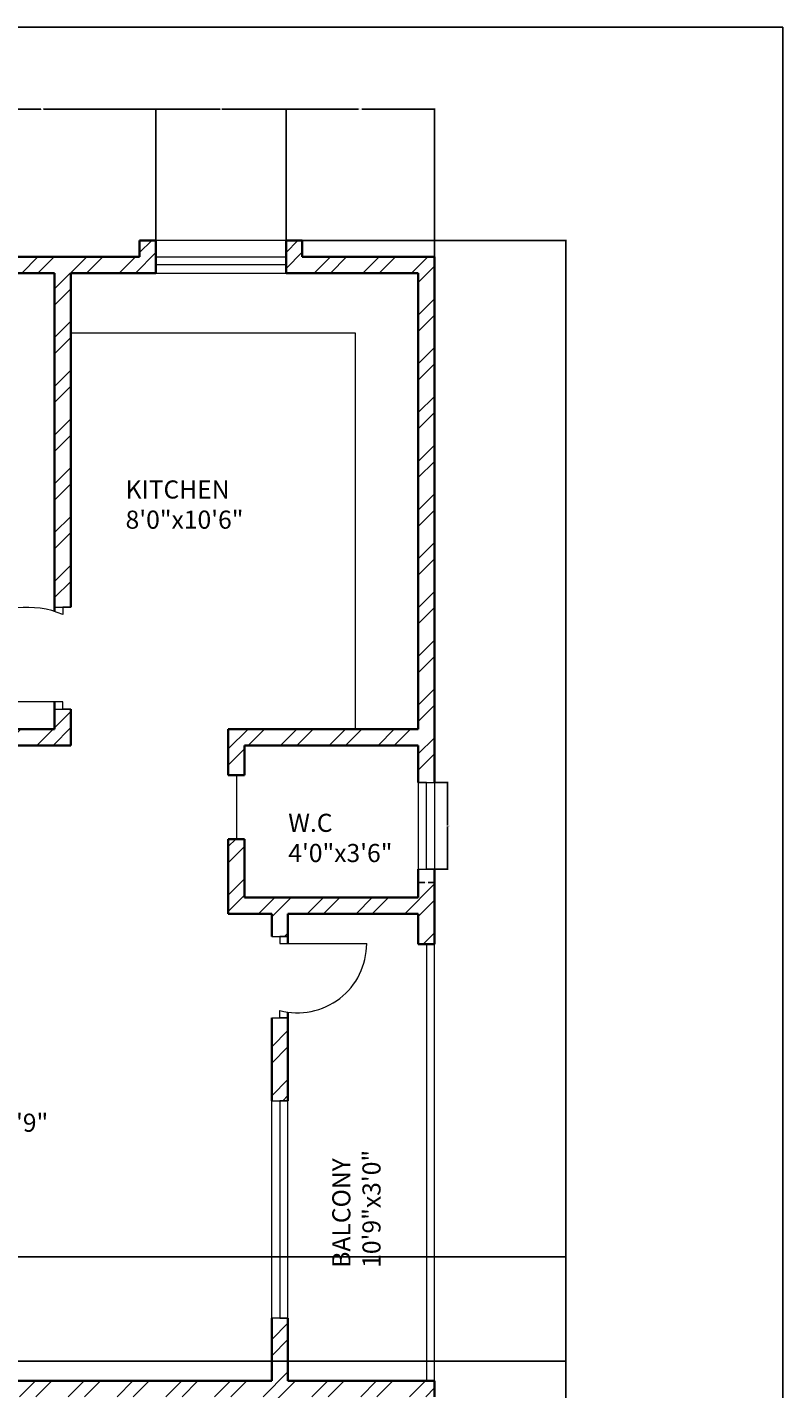
# Model space of a CAD drawing. Units: inches. Extents: x 1570 to 2186, y 1575 to 2421.
# Tile 10 of 10: x 1978 to 2186, y 2045 to 2421. Entities that reach past the tile are written whole.
import ezdxf

# ---------------------------------------------------------------- set-up
doc = ezdxf.new("R2010")
doc.units = ezdxf.units.IN
for name, color, linetype, lineweight in [('A-ANNO-DIMS', 2, 'Continuous', 18), ('A-ANNO-TTLB', 7, 'Continuous', 25), ('A-AREA-IDEN', 7, 'Continuous', 18), ('A-DOOR', 201, 'Continuous', 18), ('A-FLOR-CASE', 7, 'Continuous', 18), ('A-FLOR-HRAL', 201, 'Continuous', 18), ('A-GLAZ', 150, 'Continuous', 18), ('A-WALL', 7, 'Continuous', 35), ('A-WALL-PATT', 252, 'Continuous', 13)]:
    doc.layers.add(name, color=color, linetype=linetype, lineweight=lineweight)
doc.styles.get("Standard").update_dxf_attribs({"font": 'arial.ttf'})
doc.dimstyles.get("Standard").update_dxf_attribs({"dimtxt": 0.18, "dimasz": 0.18, "dimexe": 0.18, "dimexo": 0.0625, "dimgap": 0.09, "dimtad": 0, "dimtih": 1, "dimtoh": 1, "dimdec": 4, "dimzin": 0, "dimdsep": 46, "dimtxsty": 'Standard', "dimcen": 0.09, "dimadec": 0, "dimazin": 0, "dimtfac": 1, "dimtdec": 4, "dimtofl": 0, "dimtmove": 0, "dimatfit": 3, "dimfxl": 1, "dimtolj": 1, "dimtzin": 0, "dimarcsym": 0})

# ---------------------------------------------------------------- blocks, each defined once
blk = doc.blocks.new('WIN-24IN')
for p, q in [((2.25, 24), (0, 24)), ((0, 24), (4.5, 24)), ((0, 24), (0, 0)), ((2.25, 0), (2.25, 24)), ((4.5, 24), (4.5, 0)), ((0, 0), (4.5, 0)), ((4.5, 0), (2.25, 0))]:
    blk.add_line(p, q)
blk = doc.blocks.new('*D8')
at = {"layer": 'A-ANNO-DIMS', "color": 0, "lineweight": -2, "transparency": 16777216}
for p, q in [((2090.15, 2212.44), (2093.87, 2212.44)), ((2093.69, 2212.26), (2093.69, 2200.62)), ((2093.69, 2188.62), (2093.69, 2200.26)), ((2090.15, 2188.44), (2093.87, 2188.44))]:
    blk.add_line(p, q, dxfattribs=at)
at = {"layer": 'A-ANNO-DIMS', "color": 0, "transparency": 16777216}
for points in [[(2093.66, 2212.26), (2093.72, 2212.26), (2093.69, 2212.44)], [(2093.66, 2188.62), (2093.72, 2188.62), (2093.69, 2188.44)]]:
    blk.add_solid(points, dxfattribs=at)
at = {"layer": 'Defpoints', "color": 0, "transparency": 16777216}
for p in [(2090.09, 2212.44), (2093.69, 2212.44), (2090.09, 2188.44)]:
    blk.add_point(p, dxfattribs=at)
at = {"layer": 'A-ANNO-DIMS', "color": 0, "transparency": 16777216, "insert": (2093.69, 2200.44), "char_height": 0.18, "attachment_point": 5}
blk.add_mtext('\\A1;WINDOW 24 TYP.', dxfattribs=at)
blk = doc.blocks.new('*D9')
at = {"layer": 'A-ANNO-DIMS', "color": 0, "lineweight": -2, "transparency": 16777216}
for p, q in [((2085.59, 2188.38), (2085.59, 2184.66)), ((2090.09, 2188.38), (2090.09, 2184.66)), ((2085.77, 2184.84), (2087.38, 2184.84)), ((2089.91, 2184.84), (2088.3, 2184.84))]:
    blk.add_line(p, q, dxfattribs=at)
at = {"layer": 'A-ANNO-DIMS', "color": 0, "transparency": 16777216}
for points in [[(2085.77, 2184.87), (2085.77, 2184.81), (2085.59, 2184.84)], [(2089.91, 2184.87), (2089.91, 2184.81), (2090.09, 2184.84)]]:
    blk.add_solid(points, dxfattribs=at)
at = {"layer": 'Defpoints', "color": 0, "transparency": 16777216}
for p in [(2085.59, 2188.44), (2090.09, 2188.44), (2090.09, 2184.84)]:
    blk.add_point(p, dxfattribs=at)
at = {"layer": 'A-ANNO-DIMS', "color": 0, "transparency": 16777216, "insert": (2087.84, 2184.84), "char_height": 0.18, "attachment_point": 5}
blk.add_mtext('\\A1;5 TYP.', dxfattribs=at)
blk = doc.blocks.new('*D28')
at = {"layer": 'A-ANNO-DIMS', "color": 0, "lineweight": -2, "transparency": 16777216}
for p, q in [((1950.26, 2362.21), (1950.26, 2398.63)), ((1950.44, 2398.45), (1981.26, 2398.45)), ((2012.86, 2398.45), (1982.05, 2398.45)), ((2013.04, 2362.21), (2013.04, 2398.63))]:
    blk.add_line(p, q, dxfattribs=at)
at = {"layer": 'A-ANNO-DIMS', "color": 0, "transparency": 16777216}
for points in [[(1950.44, 2398.48), (1950.44, 2398.42), (1950.26, 2398.45)], [(2012.86, 2398.48), (2012.86, 2398.42), (2013.04, 2398.45)]]:
    blk.add_solid(points, dxfattribs=at)
at = {"layer": 'Defpoints', "color": 0, "transparency": 16777216}
for p in [(2013.04, 2398.45), (1950.26, 2362.15), (2013.04, 2362.15)]:
    blk.add_point(p, dxfattribs=at)
at = {"layer": 'A-ANNO-DIMS', "color": 0, "transparency": 16777216, "insert": (1981.65, 2398.45), "char_height": 0.18, "attachment_point": 5}
blk.add_mtext('\\A1;62.78', dxfattribs=at)
blk = doc.blocks.new('*D29')
at = {"layer": 'A-ANNO-DIMS', "color": 0, "lineweight": -2, "transparency": 16777216}
for p, q in [((2013.04, 2362.21), (2013.04, 2398.63)), ((2013.22, 2398.45), (2030.82, 2398.45)), ((2048.86, 2398.45), (2031.26, 2398.45)), ((2049.04, 2362.21), (2049.04, 2398.63))]:
    blk.add_line(p, q, dxfattribs=at)
at = {"layer": 'A-ANNO-DIMS', "color": 0, "transparency": 16777216}
for points in [[(2013.22, 2398.48), (2013.22, 2398.42), (2013.04, 2398.45)], [(2048.86, 2398.48), (2048.86, 2398.42), (2049.04, 2398.45)]]:
    blk.add_solid(points, dxfattribs=at)
at = {"layer": 'Defpoints', "color": 0, "transparency": 16777216}
for p in [(2049.04, 2398.45), (2013.04, 2362.15), (2049.04, 2362.15)]:
    blk.add_point(p, dxfattribs=at)
at = {"layer": 'A-ANNO-DIMS', "color": 0, "transparency": 16777216, "insert": (2031.04, 2398.45), "char_height": 0.18, "attachment_point": 5}
blk.add_mtext('\\A1;36', dxfattribs=at)
blk = doc.blocks.new('*D30')
at = {"layer": 'A-ANNO-DIMS', "color": 0, "lineweight": -2, "transparency": 16777216}
for p, q in [((2049.04, 2362.21), (2049.04, 2398.63)), ((2049.22, 2398.45), (2069.1, 2398.45)), ((2089.91, 2398.45), (2070.03, 2398.45)), ((2090.09, 2357.71), (2090.09, 2398.63))]:
    blk.add_line(p, q, dxfattribs=at)
at = {"layer": 'A-ANNO-DIMS', "color": 0, "transparency": 16777216}
for points in [[(2049.22, 2398.48), (2049.22, 2398.42), (2049.04, 2398.45)], [(2089.91, 2398.48), (2089.91, 2398.42), (2090.09, 2398.45)]]:
    blk.add_solid(points, dxfattribs=at)
at = {"layer": 'Defpoints', "color": 0, "transparency": 16777216}
for p in [(2090.09, 2398.45), (2049.04, 2362.15), (2090.09, 2357.65)]:
    blk.add_point(p, dxfattribs=at)
at = {"layer": 'A-ANNO-DIMS', "color": 0, "transparency": 16777216, "insert": (2069.57, 2398.45), "char_height": 0.18, "attachment_point": 5}
blk.add_mtext('\\A1;41.045', dxfattribs=at)
blk = doc.blocks.new('*D32')
at = {"layer": 'A-ANNO-DIMS', "color": 0, "lineweight": -2, "transparency": 16777216}
for p, q in [((2053.61, 2362.15), (2126.57, 2362.15)), ((2126.39, 2361.97), (2126.39, 2042.13)), ((2126.39, 1721.93), (2126.39, 2041.77)), ((2058.81, 1721.75), (2126.57, 1721.75))]:
    blk.add_line(p, q, dxfattribs=at)
at = {"layer": 'A-ANNO-DIMS', "color": 0, "transparency": 16777216}
for points in [[(2126.36, 2361.97), (2126.42, 2361.97), (2126.39, 2362.15)], [(2126.36, 1721.93), (2126.42, 1721.93), (2126.39, 1721.75)]]:
    blk.add_solid(points, dxfattribs=at)
at = {"layer": 'Defpoints', "color": 0, "transparency": 16777216}
for p in [(2053.54, 2362.15), (2126.39, 2362.15), (2058.75, 1721.75)]:
    blk.add_point(p, dxfattribs=at)
at = {"layer": 'A-ANNO-DIMS', "color": 0, "transparency": 16777216, "insert": (2126.39, 2041.95), "char_height": 0.18, "attachment_point": 5}
blk.add_mtext('\\A1;640.4', dxfattribs=at)
blk = doc.blocks.new('*D40')
at = {"layer": 'A-ANNO-DIMS', "color": 0, "lineweight": -2, "transparency": 16777216}
for p, q in [((1816.15, 2081.37), (2126.57, 2081.37)), ((2126.39, 2081.19), (2126.39, 2067.15)), ((2126.39, 2052.75), (2126.39, 2066.79)), ((1816.15, 2052.57), (2126.57, 2052.57))]:
    blk.add_line(p, q, dxfattribs=at)
at = {"layer": 'A-ANNO-DIMS', "color": 0, "transparency": 16777216}
for points in [[(2126.36, 2081.19), (2126.42, 2081.19), (2126.39, 2081.37)], [(2126.36, 2052.75), (2126.42, 2052.75), (2126.39, 2052.57)]]:
    blk.add_solid(points, dxfattribs=at)
at = {"layer": 'Defpoints', "color": 0, "transparency": 16777216}
for p in [(1816.09, 2081.37), (2126.39, 2081.37), (1816.09, 2052.57)]:
    blk.add_point(p, dxfattribs=at)
at = {"layer": 'A-ANNO-DIMS', "color": 0, "transparency": 16777216, "insert": (2126.39, 2066.97), "char_height": 0.18, "attachment_point": 5}
blk.add_mtext('\\A1;28.8', dxfattribs=at)

msp = doc.modelspace()

# ---------------------------------------------------------------- hatches: boundary and pattern name
at = {"layer": 'A-WALL-PATT'}
h = msp.add_hatch(dxfattribs=at)
h.set_pattern_fill('ANSI32', color=256)
h.paths.add_polyline_path([(1762.0975, 2362.1492), (1757.5975, 2362.1492), (1757.5975, 2357.6492), (1709.1163, 2357.6492), (1709.1163, 2362.1492), (1704.6163, 2362.1492), (1704.6163, 2353.1492), (1740.0886, 2353.1492), (1740.0886, 2261.8115), (1744.5886, 2261.8115), (1744.5886, 2353.1492), (1762.0975, 2353.1492)])
h.paths.add_polyline_path([(1890.2592, 2362.1492), (1885.7592, 2362.1492), (1826.5975, 2362.1492), (1822.0975, 2362.1492), (1822.0975, 2353.1492), (1862.5886, 2353.1492), (1862.5886, 2227.1492), (1744.5886, 2227.1492), (1744.5886, 2229.5389), (1742.3386, 2229.5389), (1740.0886, 2229.5389), (1740.0886, 2222.6492), (1744.5886, 2222.6492), (1756.186, 2222.6492), (1756.186, 2216.3571), (1760.686, 2216.3571), (1760.686, 2222.6492), (1832.686, 2222.6492), (1832.686, 2212.5994), (1837.186, 2212.5994), (1837.186, 2222.6492), (1893.186, 2222.6492), (1893.186, 2212.5994), (1897.686, 2212.5994), (1897.686, 2222.6492), (1989.5886, 2222.6492), (1989.5886, 2227.1492), (1989.5886, 2232.6585), (1987.3386, 2232.6585), (1985.0886, 2232.6585), (1985.0886, 2227.1492), (1867.0886, 2227.1492), (1867.0886, 2353.1492), (1890.2592, 2353.1492)])
h.paths.add_polyline_path([(1644.0886, 2353.1492), (1668.6163, 2353.1492), (1668.6163, 2362.1492), (1664.1163, 2362.1492), (1664.1163, 2358.9932), (1664.1163, 2357.6492), (1639.5886, 2357.6492), (1639.5886, 2213.8746), (1644.0886, 2213.8746), (1644.0886, 2222.6492), (1692.0886, 2222.6492), (1692.0886, 2215.9343), (1696.5886, 2215.9343), (1696.5886, 2222.6492), (1696.5886, 2227.1492), (1644.0886, 2227.1492)])
h.paths.add_polyline_path([(2013.0435, 2362.1492), (2008.5435, 2362.1492), (2008.5435, 2357.6492), (1954.7592, 2357.6492), (1954.7592, 2362.1492), (1950.2592, 2362.1492), (1950.2592, 2353.1492), (1985.0886, 2353.1492), (1985.0886, 2260.8534), (1989.5886, 2260.8534), (1989.5886, 2353.1492), (2013.0435, 2353.1492)])
h.paths.add_polyline_path([(2090.0886, 2357.6492), (2053.5435, 2357.6492), (2053.5435, 2362.1492), (2049.0435, 2362.1492), (2049.0435, 2353.1492), (2085.5886, 2353.1492), (2085.5886, 2227.1492), (2033.0886, 2227.1492), (2033.0886, 2222.6492), (2033.0886, 2214.4464), (2037.5886, 2214.4464), (2037.5886, 2222.6492), (2085.5886, 2222.6492), (2085.5886, 2212.4409), (2090.0886, 2212.4409)])
h.paths.add_polyline_path([(2090.0886, 2188.4409), (2087.8386, 2188.4409), (2085.5886, 2188.4409), (2085.5886, 2180.6492), (2037.5886, 2180.6492), (2037.5886, 2196.7956), (2033.0886, 2196.7956), (2033.0886, 2176.1492), (2037.5886, 2176.1492), (2045.0886, 2176.1492), (2045.0886, 2169.8988), (2049.5886, 2169.8988), (2049.5886, 2176.1492), (2085.5886, 2176.1492), (2085.5886, 2167.785), (2090.0886, 2167.785)])
h.paths.add_polyline_path([(2049.5886, 2147.4502), (2047.3386, 2147.4502), (2045.0886, 2147.4502), (2045.0886, 2124.4703), (2049.5886, 2124.4703)])
h.paths.add_polyline_path([(2090.0886, 2047.1492), (2049.5886, 2047.1492), (2049.5886, 2064.4703), (2045.0886, 2064.4703), (2045.0886, 2047.1492), (1918.0886, 2047.1492), (1918.0886, 2051.2061), (1913.5886, 2051.2061), (1913.5886, 2047.1492), (1913.5886, 2036.6872), (1918.0886, 2036.6872), (1918.0886, 2042.7492), (2045.0886, 2042.7492), (2045.0886, 2027.0686), (2049.5886, 2027.0686), (2049.5886, 2042.7492), (2090.0886, 2042.7492)])
h.paths.add_polyline_path([(1918.0886, 2005.9338), (1915.8386, 2005.9338), (1913.5886, 2005.9338), (1913.5886, 1913.7492), (1918.0886, 1913.7492)])
h.paths.add_polyline_path([(2090.0886, 1913.7492), (2049.5886, 1913.7492), (2045.0886, 1913.7492), (2033.0886, 1913.7492), (2033.0886, 1909.2492), (2033.0886, 1900.9803), (2037.5886, 1900.9803), (2037.5886, 1909.2492), (2085.5886, 1909.2492), (2085.5886, 1861.2492), (2037.5886, 1861.2492), (2037.5886, 1880.0859), (2033.0886, 1880.0859), (2033.0886, 1856.7492), (2085.5886, 1856.7492), (2085.5886, 1730.7492), (2054.2483, 1730.7492), (2054.2483, 1721.7492), (2058.7483, 1721.7492), (2058.7483, 1726.2492), (2090.0886, 1726.2492)])
h.paths.add_polyline_path([(2049.5886, 1967.0686), (2045.0886, 1967.0686), (2045.0886, 1913.7492), (2049.5886, 1913.7492)])
h.paths.add_polyline_path([(1989.5886, 1824.1695), (1987.3386, 1824.1695), (1985.0886, 1824.1695), (1985.0886, 1730.7492), (1989.5886, 1730.7492)])
h.paths.add_polyline_path([(1989.5886, 1861.2492), (1974.9963, 1861.2492), (1974.9963, 1865.9306), (1972.7463, 1865.9306), (1970.4963, 1865.9306), (1970.4963, 1861.2492), (1898.4963, 1861.2492), (1898.4963, 1874.2999), (1893.9963, 1874.2999), (1893.9963, 1861.2492), (1890.5886, 1861.2492), (1837.9963, 1861.2492), (1837.9963, 1874.3159), (1833.4963, 1874.3159), (1833.4963, 1861.2492), (1761.4963, 1861.2492), (1761.4963, 1865.0209), (1759.2463, 1865.0209), (1756.9963, 1865.0209), (1756.9963, 1861.2492), (1740.0886, 1861.2492), (1740.0886, 1856.7492), (1740.0886, 1850.7206), (1744.5886, 1850.7206), (1744.5886, 1856.7492), (1985.0886, 1856.7492), (1985.0886, 1851.0804), (1989.5886, 1851.0804), (1989.5886, 1856.7492)])
h.paths.add_polyline_path([(1989.5886, 1913.7492), (1740.0886, 1913.7492), (1740.0886, 1909.2492), (1756.9963, 1909.2492), (1756.9963, 1890.279), (1761.4963, 1890.279), (1761.4963, 1909.2492), (1833.4963, 1909.2492), (1833.4963, 1898.3159), (1837.9963, 1898.3159), (1837.9963, 1909.2492), (1890.5886, 1909.2492), (1893.9963, 1909.2492), (1893.9963, 1898.2999), (1898.4963, 1898.2999), (1898.4963, 1909.2492), (1970.4963, 1909.2492), (1970.4963, 1886.9887), (1974.9963, 1886.9887), (1974.9963, 1909.2492), (1989.5886, 1909.2492)])
h.paths.add_polyline_path([(1893.7344, 1730.7492), (1867.0886, 1730.7492), (1867.0886, 1856.7492), (1862.5886, 1856.7492), (1862.5886, 1730.7492), (1824.0492, 1730.7492), (1824.0492, 1721.7492), (1893.7344, 1721.7492)])
h.paths.add_polyline_path([(2018.2483, 1730.7492), (1953.7344, 1730.7492), (1953.7344, 1721.7492), (1958.2344, 1721.7492), (1958.2344, 1726.2492), (2013.7483, 1726.2492), (2013.7483, 1721.7492), (2018.2483, 1721.7492)])
h.paths.add_polyline_path([(1768.5492, 1730.7492), (1764.0492, 1730.7492), (1744.5886, 1730.7492), (1744.5886, 1819.4364), (1742.3386, 1819.4364), (1740.0886, 1819.4364), (1740.0886, 1730.7492), (1697.3801, 1730.7492), (1697.3801, 1721.7492), (1701.8801, 1721.7492), (1701.8801, 1726.2492), (1764.0492, 1726.2492), (1764.0492, 1721.7492), (1768.5492, 1721.7492)])
h.paths.add_polyline_path([(1644.0886, 1856.7492), (1639.5886, 1856.7492), (1639.5886, 1726.2492), (1657.0315, 1726.2492), (1657.0315, 1721.7492), (1661.3801, 1721.7492), (1661.3801, 1730.7492), (1644.0886, 1730.7492)])
h.paths.add_polyline_path([(1696.5886, 1876.1809), (1692.0886, 1876.1809), (1692.0886, 1861.2492), (1684.5886, 1861.2492), (1644.0886, 1861.2492), (1644.0886, 1909.2492), (1692.0886, 1909.2492), (1692.0886, 1900.3394), (1696.5886, 1900.3394), (1696.5886, 1913.7492), (1684.5886, 1913.7492), (1684.5886, 1920.2115), (1682.3386, 1920.2115), (1680.0886, 1920.2115), (1680.0886, 1913.7492), (1639.5886, 1913.7492), (1639.5886, 1856.7492), (1684.5886, 1856.7492), (1692.0886, 1856.7492), (1696.5886, 1856.7492)])
h.paths.add_polyline_path([(1684.5886, 2042.7492), (1811.5886, 2042.7492), (1811.5886, 2038.2991), (1816.0886, 2038.2991), (1816.0886, 2042.7492), (1816.0886, 2052.5708), (1813.8386, 2052.5708), (1811.5886, 2052.5708), (1811.5886, 2047.1492), (1684.5886, 2047.1492), (1684.5886, 2064.4703), (1680.0886, 2064.4703), (1680.0886, 2047.1492), (1639.5886, 2047.1492), (1639.5886, 2042.7492), (1680.0886, 2042.7492), (1680.0886, 2024.0762), (1684.5886, 2024.0762)])
h.paths.add_polyline_path([(1684.5886, 1964.0762), (1680.0886, 1964.0762), (1680.0886, 1944.6145), (1684.5886, 1944.6145)])
h.paths.add_polyline_path([(1816.0886, 1973.7492), (1876.0886, 1973.7492), (1876.0886, 1959.17), (1880.5886, 1959.17), (1880.5886, 1973.7492), (1880.5886, 1978.2492), (1816.0886, 1978.2492), (1816.0886, 2005.9338), (1813.8386, 2005.9338), (1811.5886, 2005.9338), (1811.5886, 1913.7492), (1816.0886, 1913.7492)])
h.paths.add_polyline_path([(1837.186, 2180.6492), (1837.186, 2188.5994), (1834.936, 2188.5994), (1832.686, 2188.5994), (1832.686, 2180.6492), (1760.686, 2180.6492), (1760.686, 2197.4807), (1756.186, 2197.4807), (1756.186, 2180.6492), (1744.5886, 2180.6492), (1740.0886, 2180.6492), (1740.0886, 2176.1492), (1837.186, 2176.1492)])
h.paths.add_polyline_path([(1974.186, 2196.8744), (1971.936, 2196.8744), (1969.686, 2196.8744), (1969.686, 2180.6492), (1897.686, 2180.6492), (1897.686, 2188.5994), (1895.436, 2188.5994), (1893.186, 2188.5994), (1893.186, 2180.6492), (1893.186, 2176.1492), (1974.186, 2176.1492)])
h.paths.add_polyline_path([(1918.0886, 2176.1492), (1913.5886, 2176.1492), (1913.5886, 2081.3709), (1918.0886, 2081.3709)])
h.paths.add_polyline_path([(1816.0886, 2176.1492), (1811.5886, 2176.1492), (1811.5886, 2081.3709), (1816.0886, 2081.3709)])
h.paths.add_polyline_path([(1684.5886, 2150.4939), (1682.3386, 2150.4939), (1680.0886, 2150.4939), (1680.0886, 2124.4703), (1684.5886, 2124.4703)])
h.paths.add_polyline_path([(1696.5886, 2180.6492), (1696.5886, 2197.4701), (1692.0886, 2197.4701), (1692.0886, 2180.6492), (1644.0886, 2180.6492), (1644.0886, 2189.8746), (1641.8386, 2189.8746), (1639.5886, 2189.8746), (1639.5886, 2169.814), (1644.0886, 2169.814), (1644.0886, 2176.1492), (1680.0886, 2176.1492), (1680.0886, 2171.7002), (1684.5886, 2171.7002), (1684.5886, 2176.1492), (1696.5886, 2176.1492)])

# ---------------------------------------------------------------- linework, layer by layer
at = {"layer": 'A-ANNO-TTLB'}
msp.add_lwpolyline([(1569.8198, 2421.0436), (2186.3437, 2421.0436), (2186.3437, 1574.5084), (1569.8198, 1574.5084)], close=True, dxfattribs=at)
at = {"layer": 'A-DOOR'}
for p, q in [((1985.0886, 2260.8534), (1989.5886, 2260.8534)), ((1989.5886, 2260.8534), (1987.3386, 2260.8534)), ((1987.3386, 2260.8534), (1987.3386, 2258.8534)), ((1987.3386, 2234.6585), (1951.3386, 2234.6585)), ((1987.3386, 2232.6585), (1987.3386, 2234.6585)), ((1985.0886, 2232.6585), (1989.5886, 2232.6585)), ((1989.5886, 2232.6585), (1987.3386, 2232.6585)), ((2035.3386, 2214.4464), (2035.3386, 2196.7956)), ((2045.0886, 2169.8988), (2049.5886, 2169.8988)), ((2049.5886, 2169.8988), (2047.3386, 2169.8988)), ((2047.3386, 2169.8988), (2047.3386, 2167.8988)), ((2047.3386, 2167.8988), (2071.3386, 2167.8988)), ((2047.3386, 2147.4502), (2047.3386, 2149.4502)), ((2045.0886, 2147.4502), (2049.5886, 2147.4502)), ((2049.5886, 2147.4502), (2047.3386, 2147.4502))]:
    msp.add_line(p, q, dxfattribs=at)
for centre, radius, start, end in [((1977.4691, 2234.6585), 26.1305, 67.808551, 180), ((2052.248, 2167.8988), 19.0906, 255.098348, 0)]:
    msp.add_arc(centre, radius, start, end, dxfattribs=at)
at = {"layer": 'A-FLOR-CASE'}
for p, q in [((2068.2565, 2336.5115), (1989.5886, 2336.5115)), ((2068.2565, 2227.1492), (2068.2565, 2336.5115))]:
    msp.add_line(p, q, dxfattribs=at)
at = {"layer": 'A-FLOR-HRAL'}
for p, q in [((2087.8386, 2167.785), (2087.8386, 2047.1492)), ((2090.0886, 2047.1492), (2090.0886, 2167.785))]:
    msp.add_line(p, q, dxfattribs=at)
at = {"layer": 'A-GLAZ'}
for p, q in [((2049.0435, 2362.1492), (2013.0435, 2362.1492)), ((2013.0435, 2357.6492), (2049.0435, 2357.6492)), ((2049.0435, 2355.4238), (2013.0435, 2355.4238)), ((2013.0435, 2353.1492), (2049.0435, 2353.1492)), ((2045.0886, 2124.4703), (2049.5886, 2124.4703)), ((2045.0886, 2064.4703), (2045.0886, 2124.4703)), ((2049.5886, 2124.4703), (2047.3386, 2124.4703)), ((2047.3386, 2124.4703), (2047.3386, 2064.4703)), ((2049.5886, 2064.4703), (2049.5886, 2124.4703)), ((2049.5886, 2064.4703), (2045.0886, 2064.4703)), ((2047.3386, 2064.4703), (2049.5886, 2064.4703))]:
    msp.add_line(p, q, dxfattribs=at)
at = {"layer": 'A-WALL'}
for p, q in [((2013.0435, 2362.1492), (2008.5435, 2362.1492)), ((2008.5435, 2362.1492), (2008.5435, 2357.6492)), ((2008.5435, 2362.1492), (2013.0435, 2362.1492)), ((2013.0435, 2353.1492), (2013.0435, 2362.1492)), ((2049.0435, 2353.1492), (2049.0435, 2362.1492)), ((2049.0435, 2362.1492), (2053.5435, 2362.1492)), ((2053.5435, 2362.1492), (2053.5435, 2357.6492)), ((1954.7592, 2357.6492), (2008.5435, 2357.6492)), ((2053.5435, 2357.6492), (2090.0886, 2357.6492)), ((2090.0886, 2357.6492), (2090.0886, 2212.4409)), ((1950.2592, 2353.1492), (1985.0886, 2353.1492)), ((1985.0886, 2353.1492), (1985.0886, 2259.6534)), ((1989.5886, 2353.1492), (1989.5886, 2260.8534)), ((1989.5886, 2353.1492), (2013.0435, 2353.1492)), ((2049.0435, 2353.1492), (2085.5886, 2353.1492)), ((2085.5886, 2353.1492), (2085.5886, 2227.1492)), ((1985.0886, 2234.6585), (1985.0886, 2227.1492)), ((1989.5886, 2232.6585), (1989.5886, 2227.1492)), ((1867.0886, 2227.1492), (1985.0886, 2227.1492)), ((1989.5886, 2227.1492), (1989.5886, 2222.6492)), ((2033.0886, 2227.1492), (2085.5886, 2227.1492)), ((2033.0886, 2222.6492), (2033.0886, 2227.1492)), ((1897.686, 2222.6492), (1989.5886, 2222.6492)), ((2033.0886, 2214.4464), (2033.0886, 2222.6492)), ((2037.5886, 2222.6492), (2037.5886, 2214.4464)), ((2037.5886, 2222.6492), (2085.5886, 2222.6492)), ((2085.5886, 2222.6492), (2085.5886, 2212.4409)), ((2037.5886, 2214.4464), (2033.0886, 2214.4464)), ((2033.0886, 2176.1492), (2033.0886, 2196.7956)), ((2033.0886, 2196.7956), (2037.5886, 2196.7956)), ((2037.5886, 2196.7956), (2037.5886, 2180.6492)), ((2085.5886, 2188.4409), (2085.5886, 2180.6492)), ((2090.0886, 2188.4409), (2090.0886, 2167.785)), ((2037.5886, 2180.6492), (2085.5886, 2180.6492)), ((2037.5886, 2176.1492), (2033.0886, 2176.1492)), ((2045.0886, 2176.1492), (2037.5886, 2176.1492)), ((2045.0886, 2176.1492), (2045.0886, 2169.8988)), ((2085.5886, 2176.1492), (2049.5886, 2176.1492)), ((2049.5886, 2176.1492), (2049.5886, 2167.8988)), ((2085.5886, 2176.1492), (2085.5886, 2167.785)), ((2085.5886, 2167.785), (2090.0886, 2167.785)), ((2049.5886, 2148.9943), (2049.5886, 2124.4703)), ((2045.0886, 2147.4502), (2045.0886, 2124.4703)), ((2045.0886, 2064.4703), (2045.0886, 2047.1492)), ((2049.5886, 2064.4703), (2049.5886, 2047.1492)), ((2045.0886, 2047.1492), (1918.0886, 2047.1492)), ((2045.0886, 2047.1492), (1918.0886, 2047.1492)), ((2045.0886, 2047.1492), (2037.5886, 2047.1492)), ((2090.0886, 2047.1492), (2049.5886, 2047.1492)), ((2090.0886, 2047.1492), (2090.0886, 2042.7492))]:
    msp.add_line(p, q, dxfattribs=at)

# ---------------------------------------------------------------- block references
at = {"layer": 'A-GLAZ'}
msp.add_blockref('WIN-24IN', (2085.589, 2188.441), dxfattribs=at)

# ---------------------------------------------------------------- texts
at = {"layer": 'A-AREA-IDEN', "char_height": 5, "attachment_point": 1}
for s, width, insert in [('KITCHEN\\P8\'0"x10\'6"', 180.522731, (2004.6937, 2295.8567)), ('W.C \\P4\'0"x3\'6"', 83.627588, (2049.6578, 2203.7767)), ('LIVING\\P10\'7"x10\'9"', 308.463782, (1946.9462, 2129.2788))]:
    msp.add_mtext_dynamic_manual_height_columns(s, width=width, gutter_width=12.5, heights=[0], dxfattribs=dict(at, insert=insert))
at = {"layer": 'A-AREA-IDEN', "insert": (2061.8302, 2078.3535), "char_height": 5, "attachment_point": 1, "rotation": 90}
msp.add_mtext_dynamic_manual_height_columns('BALCONY\\P10\'9"x3\'0"', width=143.500935, gutter_width=12.5, heights=[0], dxfattribs=at)

# ---------------------------------------------------------------- dimensions: what is measured, and where the dimension line sits
at = {"layer": 'A-ANNO-DIMS'}
for base, p1, p2, override, picture, middle in [((2013.0435, 2398.4492), (1950.2592, 2362.1492), (2013.0435, 2362.1492), {"dimdec": 2, "dimlfac": 1, "dimrnd": 0, "dimzin": 0, "dimdsep": 46, "dimlunit": 2}, '*D28', (1981.6513, 2398.4492)), ((2049.0435, 2398.4492), (2013.0435, 2362.1492), (2049.0435, 2362.1492), {"dimdec": 0, "dimlfac": 1, "dimrnd": 0, "dimzin": 0, "dimdsep": 46, "dimlunit": 2}, '*D29', (2031.0435, 2398.4492)), ((2090.0886, 2398.4492), (2049.0435, 2362.1492), (2090.0886, 2357.6492), {"dimdec": 3, "dimlfac": 1, "dimrnd": 0, "dimzin": 0, "dimdsep": 46, "dimlunit": 2}, '*D30', (2069.566, 2398.4492))]:
    dim = msp.add_linear_dim(base=base, p1=p1, p2=p2, dimstyle='Standard', override=override, dxfattribs=at)
    dim.commit()
    dim.dimension.update_dxf_attribs({"geometry": picture, "text_midpoint": middle})
for base, p1, p2, picture, middle in [((2126.3886, 2362.1492), (2058.7483, 1721.7492), (2053.5435, 2362.1492), '*D32', (2126.3886, 2041.9492)), ((2126.3886, 2081.3709), (1816.0886, 2052.5708), (1816.0886, 2081.3709), '*D40', (2126.3886, 2066.9709))]:
    dim = msp.add_linear_dim(base=base, p1=p1, p2=p2, angle=90, dimstyle='Standard', override={"dimdec": 1, "dimlfac": 1, "dimrnd": 0, "dimzin": 0, "dimdsep": 46, "dimlunit": 2}, dxfattribs=at)
    dim.commit()
    dim.dimension.update_dxf_attribs({"geometry": picture, "text_midpoint": middle})
dim = msp.add_linear_dim(base=(2093.6886, 2212.4409), p1=(2090.0886, 2188.4409), p2=(2090.0886, 2212.4409), angle=90, text='WINDOW <> TYP.', dimstyle='Standard', override={"dimdec": 0, "dimlfac": 1, "dimrnd": 0, "dimzin": 0, "dimdsep": 46, "dimlunit": 2}, dxfattribs=at)
dim.commit()
dim.dimension.update_dxf_attribs({"geometry": '*D8', "text_midpoint": (2093.6886, 2200.4409)})
dim = msp.add_linear_dim(base=(2090.0886393898, 2184.8408716997), p1=(2085.5886393898, 2188.4408716997), p2=(2090.0886393898, 2188.4408716997), text='<> TYP.', dimstyle='Standard', override={"dimdec": 0, "dimlfac": 1, "dimrnd": 0, "dimzin": 0, "dimdsep": 46, "dimlunit": 2}, dxfattribs=at)
dim.commit()
dim.dimension.update_dxf_attribs({"geometry": '*D9', "text_midpoint": (2087.8386393898, 2184.8408716997)})

doc.saveas('drawing.dxf')
